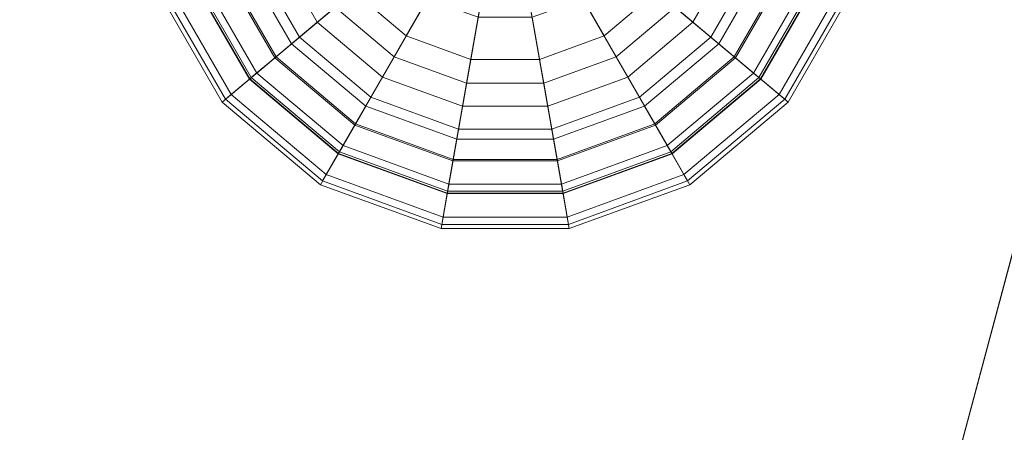
# Model space of a CAD drawing. Units: inches. Extents: x 375 to 1122, y 27 to 1069.
# Tile 108 of 155: x 731.282 to 734.892, y 871.191 to 872.701. Entities that reach past the tile are written whole.
import ezdxf

# ---------------------------------------------------------------- set-up
doc = ezdxf.new("R2010")
doc.units = ezdxf.units.IN
doc.layers.add('A-ANNO-DIMS', color=2, linetype='Continuous', lineweight=18)
doc.layers.add('Furniture', color=30, linetype='Continuous', lineweight=18)
doc.styles.get("Standard").update_dxf_attribs({"font": 'arial.ttf'})
doc.dimstyles.new('ISO-25', dxfattribs={"dimtxt": 12, "dimasz": 2.5, "dimexe": 1.5, "dimexo": 1.5, "dimtad": 1, "dimdec": 1, "dimlunit": 3, "dimtxsty": 'Standard', "dimblk": 'ARCHTICK', "dimcen": 2.5, "dimadec": 0, "dimazin": 0, "dimtfac": 1, "dimtdec": 1, "dimtmove": 0, "dimatfit": 3, "dimfxl": 1.5, "dimfxlon": 1, "dimarcsym": 0})

# ---------------------------------------------------------------- blocks, each defined once
blk = doc.blocks.new('A$C403C54AD')
at = {"linetype": 'ByBlock', "invisible_edges": 5}
for points in [[(1.674179, 1.280047, -0.037345), (1.657248, 1.250721, -0.02811), (1.726512, 1.232162, -0.02811), (1.726512, 1.266024, -0.037345)], [(1.657248, 1.250721, -0.023492), (1.666483, 1.266717, -0.023492), (1.726512, 1.250632, -0.023492), (1.726512, 1.232162, -0.023492)]]:
    blk.add_3dface(points, dxfattribs=at)
at = {"linetype": 'ByBlock'}
blk.add_3dface([(1.657248, 1.250721, -0.02811), (1.657248, 1.250721, -0.023492), (1.726512, 1.232162, -0.023492), (1.726512, 1.232162, -0.02811)], dxfattribs=at)
for points in [[(1.64823, 1.228857, -0.04658), (1.626464, 1.202917, -0.043501), (1.626464, 1.202917, -0.043501), (1.638046, 1.234737, -0.04658)], [(1.646105, 1.226325, 0.116404), (1.647974, 1.228552, 0.10318), (1.637909, 1.234363, 0.10318), (1.636915, 1.231631, 0.116404)], [(1.646131, 1.226356, -0.043349), (1.64823, 1.228857, -0.04658), (1.638046, 1.234737, -0.04658), (1.636929, 1.231669, -0.043349)], [(1.647974, 1.228552, 0.10318), (1.64754, 1.228035, 0.074938), (1.637678, 1.233728, 0.074938), (1.637909, 1.234363, 0.10318)], [(1.64754, 1.228035, 0.074938), (1.644092, 1.223925, 0.056929), (1.635844, 1.228687, 0.056929), (1.637678, 1.233728, 0.074938)], [(1.635601, 1.213806, -0.040074), (1.646131, 1.226356, -0.043349), (1.636929, 1.231669, -0.043349), (1.631326, 1.216274, -0.040074)], [(1.642894, 1.222497, 0.12581), (1.646105, 1.226325, 0.116404), (1.636915, 1.231631, 0.116404), (1.635206, 1.226936, 0.12581)], [(1.645991, 1.226189, 0.102963), (1.644185, 1.224037, 0.115599), (1.635893, 1.228824, 0.115599), (1.636854, 1.231464, 0.102963)], [(1.645568, 1.225685, 0.075423), (1.645991, 1.226189, 0.102963), (1.636854, 1.231464, 0.102963), (1.636629, 1.230846, 0.075423)], [(1.642285, 1.221772, 0.058276), (1.645568, 1.225685, 0.075423), (1.636629, 1.230846, 0.075423), (1.634882, 1.226046, 0.058276)], [(1.65579, 1.219849, -0.04658), (1.626464, 1.202917, -0.043501), (1.626464, 1.202917, -0.043501), (1.64823, 1.228857, -0.04658)], [(1.644092, 1.223925, 0.056929), (1.63955, 1.218512, 0.046697), (1.633427, 1.222047, 0.046697), (1.635844, 1.228687, 0.056929)], [(1.644185, 1.224037, 0.115599), (1.640915, 1.220139, 0.12581), (1.634153, 1.224043, 0.12581), (1.635893, 1.228824, 0.115599)], [(1.652926, 1.218195, 0.116404), (1.655444, 1.219649, 0.10318), (1.647974, 1.228552, 0.10318), (1.646105, 1.226325, 0.116404)], [(1.652961, 1.218216, -0.043349), (1.65579, 1.219849, -0.04658), (1.64823, 1.228857, -0.04658), (1.646131, 1.226356, -0.043349)], [(1.655444, 1.219649, 0.10318), (1.65486, 1.219312, 0.074938), (1.64754, 1.228035, 0.074938), (1.647974, 1.228552, 0.10318)], [(1.65486, 1.219312, 0.074938), (1.650214, 1.216629, 0.056929), (1.644092, 1.223925, 0.056929), (1.64754, 1.228035, 0.074938)], [(1.640915, 1.220139, 0.12581), (1.642894, 1.222497, 0.12581), (1.635206, 1.226936, 0.12581), (1.634153, 1.224043, 0.12581)], [(1.638116, 1.216804, 0.048884), (1.642285, 1.221772, 0.058276), (1.634882, 1.226046, 0.058276), (1.632664, 1.219951, 0.048884)], [(1.638774, 1.210025, -0.040074), (1.652961, 1.218216, -0.043349), (1.646131, 1.226356, -0.043349), (1.635601, 1.213806, -0.040074)], [(1.648599, 1.215697, 0.12581), (1.652926, 1.218195, 0.116404), (1.646105, 1.226325, 0.116404), (1.642894, 1.222497, 0.12581)], [(1.652773, 1.218107, 0.102963), (1.65034, 1.216702, 0.115599), (1.644185, 1.224037, 0.115599), (1.645991, 1.226189, 0.102963)], [(1.652203, 1.217778, 0.075423), (1.652773, 1.218107, 0.102963), (1.645991, 1.226189, 0.102963), (1.645568, 1.225685, 0.075423)], [(1.64778, 1.215224, 0.058276), (1.652203, 1.217778, 0.075423), (1.645568, 1.225685, 0.075423), (1.642285, 1.221772, 0.058276)], [(1.65034, 1.216702, 0.115599), (1.645933, 1.214158, 0.12581), (1.640915, 1.220139, 0.12581), (1.644185, 1.224037, 0.115599)], [(1.650214, 1.216629, 0.056929), (1.644094, 1.213096, 0.046697), (1.63955, 1.218512, 0.046697), (1.644092, 1.223925, 0.056929)], [(1.645933, 1.214158, 0.12581), (1.648599, 1.215697, 0.12581), (1.642894, 1.222497, 0.12581), (1.640915, 1.220139, 0.12581)], [(1.642163, 1.211981, 0.048884), (1.64778, 1.215224, 0.058276), (1.642285, 1.221772, 0.058276), (1.638116, 1.216804, 0.048884)], [(1.659812, 1.208798, -0.04658), (1.626464, 1.202917, -0.043501), (1.626464, 1.202917, -0.043501), (1.65579, 1.219849, -0.04658)], [(1.656556, 1.208223, 0.116404), (1.659419, 1.208728, 0.10318), (1.655444, 1.219649, 0.10318), (1.652926, 1.218195, 0.116404)], [(1.656596, 1.20823, -0.043349), (1.659812, 1.208798, -0.04658), (1.65579, 1.219849, -0.04658), (1.652961, 1.218216, -0.043349)], [(1.659419, 1.208728, 0.10318), (1.658754, 1.208611, 0.074938), (1.65486, 1.219312, 0.074938), (1.655444, 1.219649, 0.10318)], [(1.658754, 1.208611, 0.074938), (1.653471, 1.20768, 0.056929), (1.650214, 1.216629, 0.056929), (1.65486, 1.219312, 0.074938)], [(1.644094, 1.213096, 0.046697), (1.635227, 1.207977, 0.03933), (1.632968, 1.210669, 0.03933), (1.63955, 1.218512, 0.046697)], [(1.640462, 1.205386, -0.040074), (1.656596, 1.20823, -0.043349), (1.652961, 1.218216, -0.043349), (1.638774, 1.210025, -0.040074)], [(1.650703, 1.207191, 0.058276), (1.655733, 1.208078, 0.075423), (1.652203, 1.217778, 0.075423), (1.64778, 1.215224, 0.058276)], [(1.651635, 1.207356, 0.12581), (1.656556, 1.208223, 0.116404), (1.652926, 1.218195, 0.116404), (1.648599, 1.215697, 0.12581)], [(1.656381, 1.208193, 0.102963), (1.653614, 1.207705, 0.115599), (1.65034, 1.216702, 0.115599), (1.652773, 1.218107, 0.102963)], [(1.655733, 1.208078, 0.075423), (1.656381, 1.208193, 0.102963), (1.652773, 1.218107, 0.102963), (1.652203, 1.217778, 0.075423)], [(1.634175, 1.207369, 0.042248), (1.642163, 1.211981, 0.048884), (1.638116, 1.216804, 0.048884), (1.632188, 1.209738, 0.042248)], [(1.653471, 1.20768, 0.056929), (1.646512, 1.206452, 0.046697), (1.644094, 1.213096, 0.046697), (1.650214, 1.216629, 0.056929)], [(1.653614, 1.207705, 0.115599), (1.648604, 1.206821, 0.12581), (1.645933, 1.214158, 0.12581), (1.65034, 1.216702, 0.115599)], [(1.644316, 1.206065, 0.048884), (1.650703, 1.207191, 0.058276), (1.64778, 1.215224, 0.058276), (1.642163, 1.211981, 0.048884)], [(1.648604, 1.206821, 0.12581), (1.651635, 1.207356, 0.12581), (1.648599, 1.215697, 0.12581), (1.645933, 1.214158, 0.12581)], [(1.646512, 1.206452, 0.046697), (1.636429, 1.204675, 0.03933), (1.635227, 1.207977, 0.03933), (1.644094, 1.213096, 0.046697)], [(1.635233, 1.204464, 0.042248), (1.644316, 1.206065, 0.048884), (1.642163, 1.211981, 0.048884), (1.634175, 1.207369, 0.042248)], [(1.659812, 1.197037, -0.04658), (1.626464, 1.202917, -0.043501), (1.626464, 1.202917, -0.043501), (1.659812, 1.208798, -0.04658)], [(1.656556, 1.197611, 0.116404), (1.659419, 1.197107, 0.10318), (1.659419, 1.208728, 0.10318), (1.656556, 1.208223, 0.116404)], [(1.656596, 1.197604, -0.043349), (1.659812, 1.197037, -0.04658), (1.659812, 1.208798, -0.04658), (1.656596, 1.20823, -0.043349)], [(1.659419, 1.197107, 0.10318), (1.658754, 1.197224, 0.074938), (1.658754, 1.208611, 0.074938), (1.659419, 1.208728, 0.10318)], [(1.640462, 1.200449, -0.040074), (1.656596, 1.197604, -0.043349), (1.656596, 1.20823, -0.043349), (1.640462, 1.205386, -0.040074)], [(1.650703, 1.198643, 0.058276), (1.655733, 1.197756, 0.075423), (1.655733, 1.208078, 0.075423), (1.650703, 1.207191, 0.058276)], [(1.651635, 1.198479, 0.12581), (1.656556, 1.197611, 0.116404), (1.656556, 1.208223, 0.116404), (1.651635, 1.207356, 0.12581)], [(1.658754, 1.197224, 0.074938), (1.653471, 1.198155, 0.056929), (1.653471, 1.20768, 0.056929), (1.658754, 1.208611, 0.074938)], [(1.656381, 1.197642, 0.102963), (1.653614, 1.19813, 0.115599), (1.653614, 1.207705, 0.115599), (1.656381, 1.208193, 0.102963)], [(1.655733, 1.197756, 0.075423), (1.656381, 1.197642, 0.102963), (1.656381, 1.208193, 0.102963), (1.655733, 1.208078, 0.075423)], [(1.644316, 1.19977, 0.048884), (1.650703, 1.198643, 0.058276), (1.650703, 1.207191, 0.058276), (1.644316, 1.206065, 0.048884)], [(1.653471, 1.198155, 0.056929), (1.646512, 1.199382, 0.046697), (1.646512, 1.206452, 0.046697), (1.653471, 1.20768, 0.056929)], [(1.653614, 1.19813, 0.115599), (1.648604, 1.199014, 0.12581), (1.648604, 1.206821, 0.12581), (1.653614, 1.207705, 0.115599)], [(1.648604, 1.199014, 0.12581), (1.651635, 1.198479, 0.12581), (1.651635, 1.207356, 0.12581), (1.648604, 1.206821, 0.12581)], [(1.635233, 1.201371, 0.042248), (1.644316, 1.19977, 0.048884), (1.644316, 1.206065, 0.048884), (1.635233, 1.204464, 0.042248)], [(1.646512, 1.199382, 0.046697), (1.636429, 1.20116, 0.03933), (1.636429, 1.204675, 0.03933), (1.646512, 1.206452, 0.046697)], [(1.65579, 1.185986, -0.04658), (1.626464, 1.202917, -0.043501), (1.626464, 1.202917, -0.043501), (1.659812, 1.197037, -0.04658)], [(1.64823, 1.176977, -0.04658), (1.626464, 1.202917, -0.043501), (1.626464, 1.202917, -0.043501), (1.65579, 1.185986, -0.04658)], [(1.638046, 1.171097, -0.04658), (1.626464, 1.202917, -0.043501), (1.626464, 1.202917, -0.043501), (1.64823, 1.176977, -0.04658)], [(1.634175, 1.198465, 0.042248), (1.642163, 1.193854, 0.048884), (1.644316, 1.19977, 0.048884), (1.635233, 1.201371, 0.042248)], [(1.644094, 1.192739, 0.046697), (1.635227, 1.197858, 0.03933), (1.636429, 1.20116, 0.03933), (1.646512, 1.199382, 0.046697)], [(1.638774, 1.19581, -0.040074), (1.652961, 1.187619, -0.043349), (1.656596, 1.197604, -0.043349), (1.640462, 1.200449, -0.040074)], [(1.642163, 1.193854, 0.048884), (1.64778, 1.190611, 0.058276), (1.650703, 1.198643, 0.058276), (1.644316, 1.19977, 0.048884)], [(1.650214, 1.189206, 0.056929), (1.644094, 1.192739, 0.046697), (1.646512, 1.199382, 0.046697), (1.653471, 1.198155, 0.056929)], [(1.645933, 1.191677, 0.12581), (1.648599, 1.190138, 0.12581), (1.651635, 1.198479, 0.12581), (1.648604, 1.199014, 0.12581)], [(1.65034, 1.189133, 0.115599), (1.645933, 1.191677, 0.12581), (1.648604, 1.199014, 0.12581), (1.653614, 1.19813, 0.115599)], [(1.632188, 1.196096, 0.042248), (1.638116, 1.189031, 0.048884), (1.642163, 1.193854, 0.048884), (1.634175, 1.198465, 0.042248)], [(1.63955, 1.187323, 0.046697), (1.632968, 1.195166, 0.03933), (1.635227, 1.197858, 0.03933), (1.644094, 1.192739, 0.046697)], [(1.64778, 1.190611, 0.058276), (1.652203, 1.188057, 0.075423), (1.655733, 1.197756, 0.075423), (1.650703, 1.198643, 0.058276)], [(1.648599, 1.190138, 0.12581), (1.652926, 1.187639, 0.116404), (1.656556, 1.197611, 0.116404), (1.651635, 1.198479, 0.12581)], [(1.65486, 1.186523, 0.074938), (1.650214, 1.189206, 0.056929), (1.653471, 1.198155, 0.056929), (1.658754, 1.197224, 0.074938)], [(1.652773, 1.187728, 0.102963), (1.65034, 1.189133, 0.115599), (1.653614, 1.19813, 0.115599), (1.656381, 1.197642, 0.102963)], [(1.652203, 1.188057, 0.075423), (1.652773, 1.187728, 0.102963), (1.656381, 1.197642, 0.102963), (1.655733, 1.197756, 0.075423)], [(1.652926, 1.187639, 0.116404), (1.655444, 1.186186, 0.10318), (1.659419, 1.197107, 0.10318), (1.656556, 1.197611, 0.116404)], [(1.652961, 1.187619, -0.043349), (1.65579, 1.185986, -0.04658), (1.659812, 1.197037, -0.04658), (1.656596, 1.197604, -0.043349)], [(1.655444, 1.186186, 0.10318), (1.65486, 1.186523, 0.074938), (1.658754, 1.197224, 0.074938), (1.659419, 1.197107, 0.10318)], [(1.635601, 1.192029, -0.040074), (1.646131, 1.179479, -0.043349), (1.652961, 1.187619, -0.043349), (1.638774, 1.19581, -0.040074)], [(1.638116, 1.189031, 0.048884), (1.642285, 1.184063, 0.058276), (1.64778, 1.190611, 0.058276), (1.642163, 1.193854, 0.048884)], [(1.644092, 1.18191, 0.056929), (1.63955, 1.187323, 0.046697), (1.644094, 1.192739, 0.046697), (1.650214, 1.189206, 0.056929)], [(1.631326, 1.18956, -0.040074), (1.636929, 1.174166, -0.043349), (1.646131, 1.179479, -0.043349), (1.635601, 1.192029, -0.040074)], [(1.640915, 1.185696, 0.12581), (1.642894, 1.183338, 0.12581), (1.648599, 1.190138, 0.12581), (1.645933, 1.191677, 0.12581)], [(1.644185, 1.181798, 0.115599), (1.640915, 1.185696, 0.12581), (1.645933, 1.191677, 0.12581), (1.65034, 1.189133, 0.115599)], [(1.642285, 1.184063, 0.058276), (1.645568, 1.18015, 0.075423), (1.652203, 1.188057, 0.075423), (1.64778, 1.190611, 0.058276)], [(1.642894, 1.183338, 0.12581), (1.646105, 1.17951, 0.116404), (1.652926, 1.187639, 0.116404), (1.648599, 1.190138, 0.12581)], [(1.632664, 1.185883, 0.048884), (1.634882, 1.179789, 0.058276), (1.642285, 1.184063, 0.058276), (1.638116, 1.189031, 0.048884)], [(1.64754, 1.1778, 0.074938), (1.644092, 1.18191, 0.056929), (1.650214, 1.189206, 0.056929), (1.65486, 1.186523, 0.074938)], [(1.645991, 1.179646, 0.102963), (1.644185, 1.181798, 0.115599), (1.65034, 1.189133, 0.115599), (1.652773, 1.187728, 0.102963)], [(1.645568, 1.18015, 0.075423), (1.645991, 1.179646, 0.102963), (1.652773, 1.187728, 0.102963), (1.652203, 1.188057, 0.075423)], [(1.635844, 1.177147, 0.056929), (1.633427, 1.183788, 0.046697), (1.63955, 1.187323, 0.046697), (1.644092, 1.18191, 0.056929)], [(1.646105, 1.17951, 0.116404), (1.647974, 1.177283, 0.10318), (1.655444, 1.186186, 0.10318), (1.652926, 1.187639, 0.116404)], [(1.646131, 1.179479, -0.043349), (1.64823, 1.176977, -0.04658), (1.65579, 1.185986, -0.04658), (1.652961, 1.187619, -0.043349)], [(1.647974, 1.177283, 0.10318), (1.64754, 1.1778, 0.074938), (1.65486, 1.186523, 0.074938), (1.655444, 1.186186, 0.10318)], [(1.634153, 1.181792, 0.12581), (1.635206, 1.178899, 0.12581), (1.642894, 1.183338, 0.12581), (1.640915, 1.185696, 0.12581)], [(1.635893, 1.177011, 0.115599), (1.634153, 1.181792, 0.12581), (1.640915, 1.185696, 0.12581), (1.644185, 1.181798, 0.115599)], [(1.634882, 1.179789, 0.058276), (1.636629, 1.174989, 0.075423), (1.645568, 1.18015, 0.075423), (1.642285, 1.184063, 0.058276)], [(1.635206, 1.178899, 0.12581), (1.636915, 1.174204, 0.116404), (1.646105, 1.17951, 0.116404), (1.642894, 1.183338, 0.12581)], [(1.637678, 1.172106, 0.074938), (1.635844, 1.177147, 0.056929), (1.644092, 1.18191, 0.056929), (1.64754, 1.1778, 0.074938)], [(1.636854, 1.174371, 0.102963), (1.635893, 1.177011, 0.115599), (1.644185, 1.181798, 0.115599), (1.645991, 1.179646, 0.102963)], [(1.636629, 1.174989, 0.075423), (1.636854, 1.174371, 0.102963), (1.645991, 1.179646, 0.102963), (1.645568, 1.18015, 0.075423)], [(1.636915, 1.174204, 0.116404), (1.637909, 1.171472, 0.10318), (1.647974, 1.177283, 0.10318), (1.646105, 1.17951, 0.116404)], [(1.636929, 1.174166, -0.043349), (1.638046, 1.171097, -0.04658), (1.64823, 1.176977, -0.04658), (1.646131, 1.179479, -0.043349)], [(1.637909, 1.171472, 0.10318), (1.637678, 1.172106, 0.074938), (1.64754, 1.1778, 0.074938), (1.647974, 1.177283, 0.10318)]]:
    blk.add_3dface(points)
blk = doc.blocks.new('_ArchTick')
at = {"color": 0, "linetype": 'ByBlock', "const_width": 0.15}
blk.add_lwpolyline([(-0.5, -0.5), (0.5, 0.5)], dxfattribs=at)
blk = doc.blocks.new('*D88')
at = {"layer": 'A-ANNO-DIMS', "color": 0, "lineweight": -2, "transparency": 16777216}
for p, q in [((731.0073, 1052.5277), (731.0073, 1055.5277)), ((854.0073, 1052.5277), (854.0073, 1055.5277)), ((731.0073, 1054.0277), (854.0073, 1054.0277))]:
    blk.add_line(p, q, dxfattribs=at)
at = {"layer": 'Defpoints', "color": 0, "transparency": 16777216}
for p in [(854.0073, 1054.0277), (731.0073, 502.5277), (854.0073, 502.5277)]:
    blk.add_point(p, dxfattribs=at)
at = {"layer": 'A-ANNO-DIMS', "color": 0, "lineweight": -2, "transparency": 16777216, "xscale": 2.5, "yscale": 2.5, "zscale": 2.5, "rotation": 180}
blk.add_blockref('_ArchTick', (731.0073, 1054.0277), dxfattribs=at)
at = {"layer": 'A-ANNO-DIMS', "color": 0, "lineweight": -2, "transparency": 16777216, "xscale": 2.5, "yscale": 2.5, "zscale": 2.5}
blk.add_blockref('_ArchTick', (854.0073, 1054.0277), dxfattribs=at)
at = {"layer": 'A-ANNO-DIMS', "color": 0, "transparency": 16777216, "insert": (792.5073, 1060.7837), "char_height": 12, "attachment_point": 5}
blk.add_mtext('10\'-3"', dxfattribs=at)
blk = doc.blocks.new('*D91')
at = {"layer": 'A-ANNO-DIMS', "color": 0, "lineweight": -2, "transparency": 16777216}
for p, q in [((728.0073, 1052.5277), (728.0073, 1055.5277)), ((788.0073, 1052.5277), (788.0073, 1055.5277)), ((728.0073, 1054.0277), (788.0073, 1054.0277))]:
    blk.add_line(p, q, dxfattribs=at)
at = {"layer": 'Defpoints', "color": 0, "transparency": 16777216}
for p in [(788.0073, 1054.0277), (728.0073, 774.0277), (788.0073, 774.0277)]:
    blk.add_point(p, dxfattribs=at)
at = {"layer": 'A-ANNO-DIMS', "color": 0, "lineweight": -2, "transparency": 16777216, "xscale": 2.5, "yscale": 2.5, "zscale": 2.5, "rotation": 180}
blk.add_blockref('_ArchTick', (728.0073, 1054.0277), dxfattribs=at)
at = {"layer": 'A-ANNO-DIMS', "color": 0, "lineweight": -2, "transparency": 16777216, "xscale": 2.5, "yscale": 2.5, "zscale": 2.5}
blk.add_blockref('_ArchTick', (788.0073, 1054.0277), dxfattribs=at)
at = {"layer": 'A-ANNO-DIMS', "color": 0, "transparency": 16777216, "insert": (758.0073, 1060.7796), "char_height": 12, "attachment_point": 5}
blk.add_mtext('5\'-0"', dxfattribs=at)

msp = doc.modelspace()

# ---------------------------------------------------------------- block references
at = {"layer": 'Furniture', "xscale": 39.9918517141215, "yscale": 39.9918517141215, "zscale": 39.9918517141215, "rotation": 270}
msp.add_blockref('A$C403C54AD', (684.9549, 938.3156, 0.024), dxfattribs=at)

# ---------------------------------------------------------------- dimensions: what is measured, and where the dimension line sits
at = {"layer": 'A-ANNO-DIMS'}
for base, p1, p2, picture, middle in [((788.0073, 1054.0277), (728.0073, 774.0277), (788.0073, 774.0277), '*D91', (758.0073, 1060.7796)), ((854.0073, 1054.0277), (731.0073, 502.5277), (854.0073, 502.5277), '*D88', (792.5073, 1060.7837))]:
    dim = msp.add_linear_dim(base=base, p1=p1, p2=p2, dimstyle='ISO-25', override={"dimdec": 1, "dimlfac": 1, "dimrnd": 0, "dimzin": 1, "dimdsep": 46, "dimlunit": 4, "dimfrac": 2}, dxfattribs=at)
    dim.commit()
    dim.dimension.update_dxf_attribs({"geometry": picture, "text_midpoint": middle})

doc.saveas('drawing.dxf')
